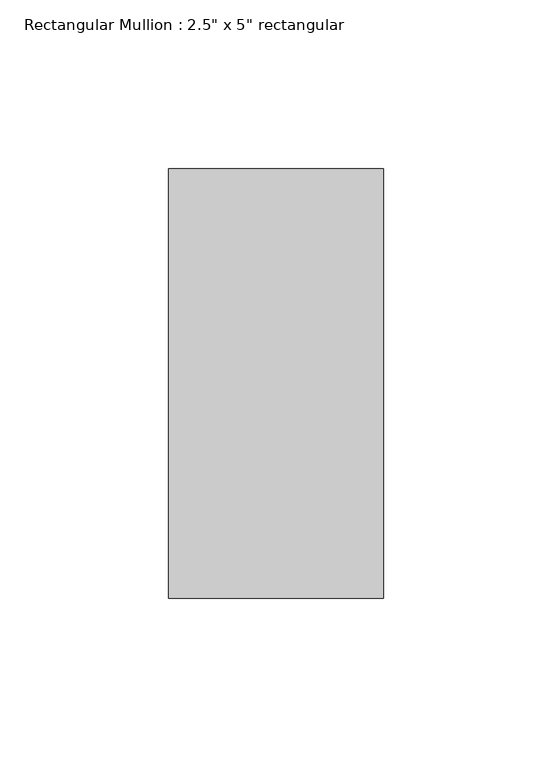
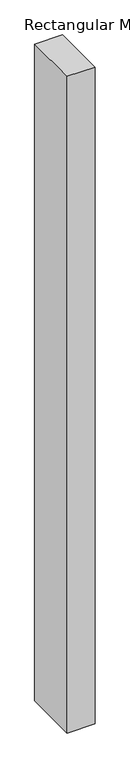
"""IFC4 building model written with IfcOpenShell, lengths in millimetres: member geometry."""

from ifc_helpers import new_model, si_unit, frame, origin, place, context, project, spatial, polyline, outline, extrude, source, transform, mapped, element, save


def member_087bde42(model_context):
    return source(origin(), model_context, "Body", "SweptSolid", [
        extrude(outline(polyline([(31.75, 63.5), (31.75, -63.5), (-31.75, -63.5), (-31.75, 63.5), (31.75, 63.5)])), frame((0.0, 0.0, -1569.5186051), z_axis=(0.0, 0.0, 1.0), x_axis=(1.0, 0.0, 0.0)), (0.0, 0.0, 1.0), 1569.5186051),
    ])


if __name__ == "__main__":
    model = new_model("IFC4")
    model_context = context("Model", 3, world=origin())
    ifc_project = project(units=[si_unit("LENGTHUNIT", "METRE", prefix="MILLI")], contexts=[model_context])
    site = spatial("IfcSite", under=ifc_project)
    building = spatial("IfcBuilding", under=site)
    placement = place(None, origin())
    member_shape = member_087bde42(model_context)
    element("IfcMember", 1, ObjectType="Rectangular Mullion : 2.5\" x 5\" rectangular", at=placement, inside=building, context=model_context, shape_type="MappedRepresentation", body=[
        mapped(member_shape, transform((0.0, 0.0, 0.0), x_axis=(1.0, 0.0, 0.0), y_axis=(0.0, 1.0, 0.0), z_axis=(0.0, 0.0, 1.0))),
    ])
    save(model, "model.ifc")

# Revit data of these elements
# Type "Rectangular Mullion : 2.5\" x 5\" rectangular"
#   built-in parameter 1007304 = 0.416667 (stored number, unit not read)
#   built-in parameter 1007301 = 0.104167 (stored number, unit not read)
#   built-in parameter 1007300 = 0.104167 (stored number, unit not read)
# Element 1 (IfcMember, "Rectangular Mullion : 2.5\" x 5\" rectangular")
#   Materials on its faces: "Aluminum"
# Materials
#   "Aluminum": class "Metal", colour RGB 247 247 247, transparency 0, Description = "Aluminum 6061", Cost = 0
